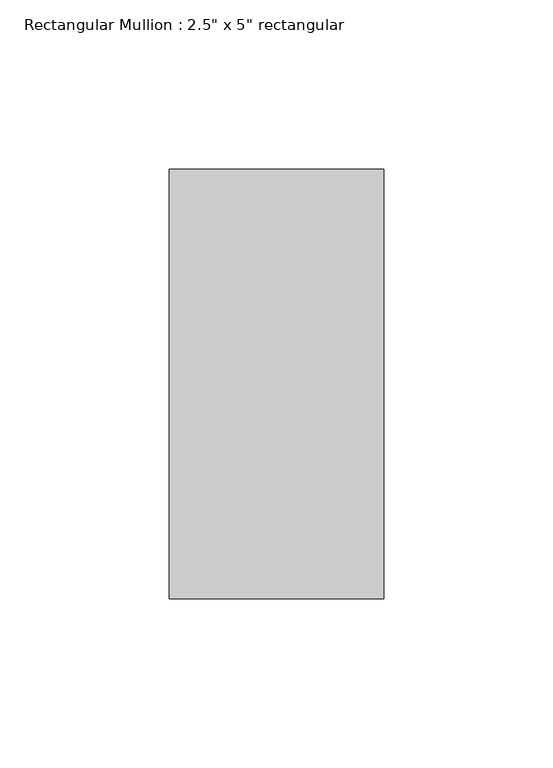
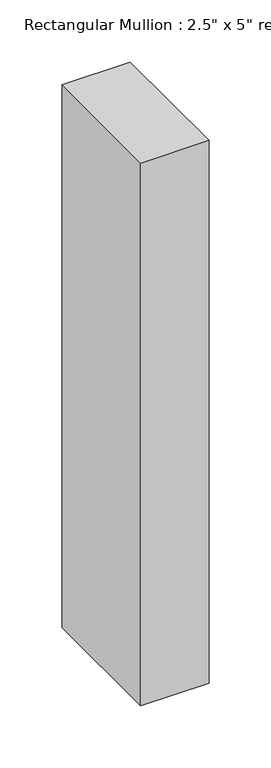
"""IFC4 building model written with IfcOpenShell, lengths in millimetres: member geometry."""

from ifc_helpers import new_model, si_unit, frame, origin, place, context, project, spatial, polyline, outline, extrude, source, transform, mapped, element, save


def member_bdfbb35d(model_context):
    return source(origin(), model_context, "Body", "SweptSolid", [
        extrude(outline(polyline([(31.75, 63.5), (31.75, -63.5), (-31.75, -63.5), (-31.75, 63.5), (31.75, 63.5)])), frame((0.0, 0.0, -533.4), z_axis=(0.0, 0.0, 1.0), x_axis=(1.0, 0.0, 0.0)), (0.0, 0.0, 1.0), 533.4),
    ])


if __name__ == "__main__":
    model = new_model("IFC4")
    model_context = context("Model", 3, world=origin())
    ifc_project = project(units=[si_unit("LENGTHUNIT", "METRE", prefix="MILLI")], contexts=[model_context])
    site = spatial("IfcSite", under=ifc_project)
    building = spatial("IfcBuilding", under=site)
    placement = place(None, origin())
    member_shape = member_bdfbb35d(model_context)
    element("IfcMember", 1, ObjectType="Rectangular Mullion : 2.5\" x 5\" rectangular", at=placement, inside=building, context=model_context, shape_type="MappedRepresentation", body=[
        mapped(member_shape, transform((0.0, 0.0, 0.0), x_axis=(1.0, 0.0, 0.0), y_axis=(0.0, 1.0, 0.0), z_axis=(0.0, 0.0, 1.0))),
    ])
    save(model, "model.ifc")

# Revit data of these elements
# Type "Rectangular Mullion : 2.5\" x 5\" rectangular"
#   built-in parameter 1007304 = 0.416667 (stored number, unit not read)
#   built-in parameter 1007301 = 0.104167 (stored number, unit not read)
#   built-in parameter 1007300 = 0.104167 (stored number, unit not read)
# Element 1 (IfcMember, "Rectangular Mullion : 2.5\" x 5\" rectangular")
#   Materials on its faces: "Aluminum"
# Materials
#   "Aluminum": class "Metal", colour RGB 247 247 247, transparency 0, Description = "Aluminum 6061", Cost = 0
